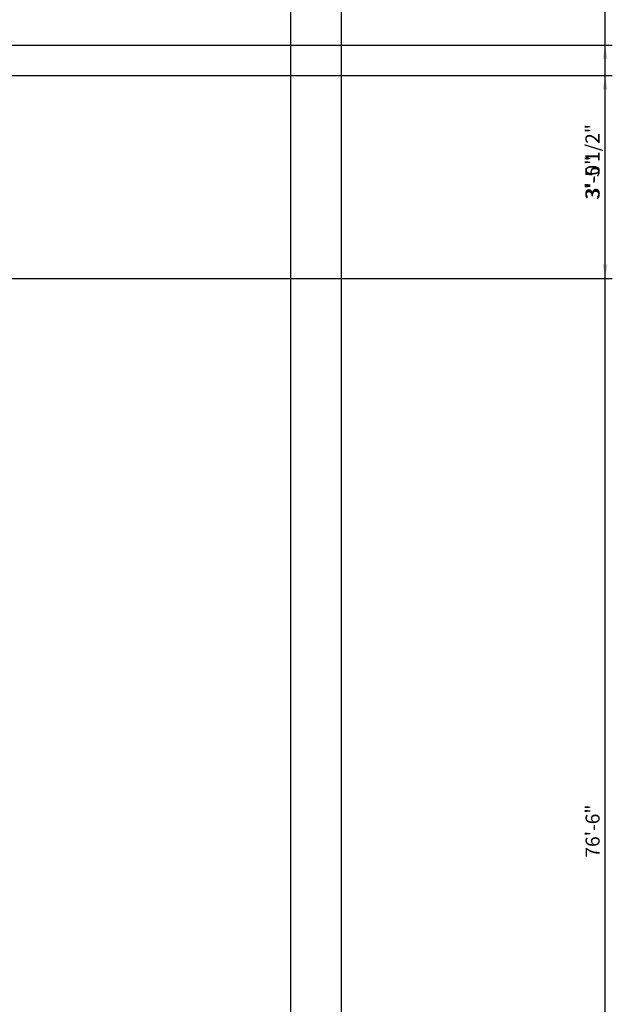
# Model space of a CAD drawing. Units: inches. Extents: x 1624 to 3956, y 1589 to 5028.
# Tile 8 of 16: x 2112 to 2218, y 2075 to 2250. Entities that reach past the tile are written whole.
import ezdxf

# ---------------------------------------------------------------- set-up
doc = ezdxf.new("R2010")
doc.units = ezdxf.units.IN
doc.layers.add('A-ANNO-DIMS', color=2, linetype='Continuous', lineweight=13)
doc.layers.add('C-PROP', color=7, linetype='Continuous', lineweight=25)
doc.styles.get("Standard").update_dxf_attribs({"font": 'arial.ttf'})
doc.dimstyles.new('Copy of ISO-25', dxfattribs={"dimtxt": 2.5, "dimasz": 2.5, "dimexe": 1.25, "dimexo": 0.625, "dimtad": 1, "dimdec": 1, "dimlunit": 4, "dimtxsty": 'Standard', "dimcen": 2.5, "dimadec": 0, "dimazin": 0, "dimtfac": 1, "dimtdec": 1, "dimtmove": 0, "dimatfit": 3, "dimfxl": 1, "dimarcsym": 0})

# ---------------------------------------------------------------- blocks, each defined once
blk = doc.blocks.new('*D67')
at = {"layer": 'A-ANNO-DIMS', "color": 0, "lineweight": -2, "transparency": 16777216}
for p, q in [((2170.2, 2564.79), (2217.63, 2564.79)), ((2216.38, 1649.29), (2216.38, 2562.29)), ((2170.2, 1646.79), (2217.63, 1646.79))]:
    blk.add_line(p, q, dxfattribs=at)
at = {"layer": 'A-ANNO-DIMS', "color": 0, "transparency": 16777216}
for points in [[(2215.96, 2562.29), (2216.8, 2562.29), (2216.38, 2564.79)], [(2215.96, 1649.29), (2216.8, 1649.29), (2216.38, 1646.79)]]:
    blk.add_solid(points, dxfattribs=at)
at = {"layer": 'Defpoints', "color": 0, "transparency": 16777216}
for p in [(2169.58, 2564.79), (2216.38, 2564.79), (2169.58, 1646.79)]:
    blk.add_point(p, dxfattribs=at)
at = {"layer": 'A-ANNO-DIMS', "color": 0, "transparency": 16777216, "insert": (2214.48, 2105.79), "char_height": 2.5, "attachment_point": 5, "rotation": 90}
blk.add_mtext('76\'-6"', dxfattribs=at)
blk = doc.blocks.new('*D80')
at = {"layer": 'A-ANNO-DIMS', "color": 0, "lineweight": -2, "transparency": 16777216}
for p, q in [((2101.2, 2245.29), (2217.63, 2245.29)), ((2216.38, 2206.34), (2216.38, 2242.79)), ((2101.2, 2203.84), (2217.63, 2203.84))]:
    blk.add_line(p, q, dxfattribs=at)
at = {"layer": 'A-ANNO-DIMS', "color": 0, "transparency": 16777216}
for points in [[(2215.96, 2242.79), (2216.8, 2242.79), (2216.38, 2245.29)], [(2215.96, 2206.34), (2216.8, 2206.34), (2216.38, 2203.84)]]:
    blk.add_solid(points, dxfattribs=at)
at = {"layer": 'Defpoints', "color": 0, "transparency": 16777216}
for p in [(2100.58, 2245.29), (2216.38, 2245.29), (2100.58, 2203.84)]:
    blk.add_point(p, dxfattribs=at)
at = {"layer": 'A-ANNO-DIMS', "color": 0, "transparency": 16777216, "insert": (2214.46, 2224.56), "char_height": 2.5, "attachment_point": 5, "rotation": 90}
blk.add_mtext('3\'-5 1/2"', dxfattribs=at)
blk = doc.blocks.new('*D95')
at = {"layer": 'A-ANNO-DIMS', "color": 0, "lineweight": -2, "transparency": 16777216}
for p, q in [((1870.18, 2239.87), (2217.63, 2239.87)), ((2216.38, 2206.37), (2216.38, 2237.37)), ((1870.18, 2203.87), (2217.63, 2203.87))]:
    blk.add_line(p, q, dxfattribs=at)
at = {"layer": 'A-ANNO-DIMS', "color": 0, "transparency": 16777216}
for points in [[(2215.96, 2237.37), (2216.8, 2237.37), (2216.38, 2239.87)], [(2215.96, 2206.37), (2216.8, 2206.37), (2216.38, 2203.87)]]:
    blk.add_solid(points, dxfattribs=at)
at = {"layer": 'Defpoints', "color": 0, "transparency": 16777216}
for p in [(1869.56, 2239.87), (2216.38, 2239.87), (1869.56, 2203.87)]:
    blk.add_point(p, dxfattribs=at)
at = {"layer": 'A-ANNO-DIMS', "color": 0, "transparency": 16777216, "insert": (2214.48, 2221.87), "char_height": 2.5, "attachment_point": 5, "rotation": 90}
blk.add_mtext('3\'-0"', dxfattribs=at)

msp = doc.modelspace()

# ---------------------------------------------------------------- linework, layer by layer
at = {"layer": 'C-PROP'}
for p, q in [((2169.58, 1652.79), (2169.58, 2559.46)), ((2160.58, 1652.79), (2160.58, 2555.79))]:
    msp.add_line(p, q, dxfattribs=at)

# ---------------------------------------------------------------- dimensions: what is measured, and where the dimension line sits
at = {"layer": 'A-ANNO-DIMS'}
for base, p1, p2, picture, middle in [((2216.38, 2564.79), (2169.58, 1646.79), (2169.58, 2564.79), '*D67', (2214.48, 2105.79)), ((2216.3792, 2245.2946), (2100.5792, 2203.8352), (2100.5792, 2245.2946), '*D80', (2214.4607, 2224.5649)), ((2216.38, 2239.87), (1869.56, 2203.87), (1869.56, 2239.87), '*D95', (2214.48, 2221.87))]:
    dim = msp.add_linear_dim(base=base, p1=p1, p2=p2, angle=90, dimstyle='Copy of ISO-25', override={"dimdec": 1, "dimlfac": 1, "dimrnd": 0, "dimzin": 1, "dimdsep": 46, "dimlunit": 4, "dimfrac": 2}, dxfattribs=at)
    dim.commit()
    dim.dimension.update_dxf_attribs({"geometry": picture, "text_midpoint": middle})

doc.saveas('drawing.dxf')
